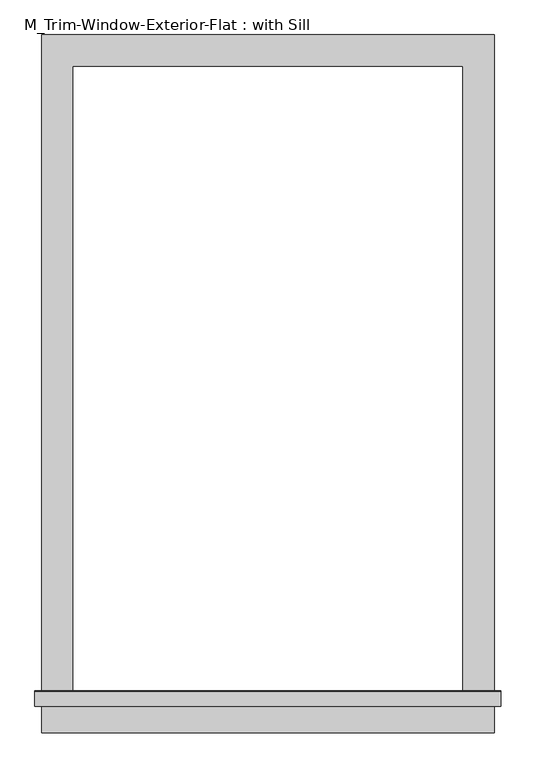
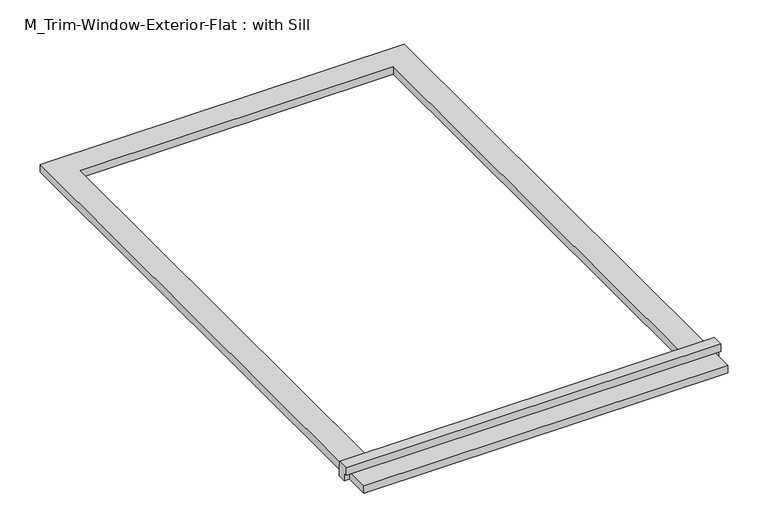
"""IFC4 building model written with IfcOpenShell, lengths in millimetres: proxy geometry, M_Trim-Window-Exterior-Flat : with Sill."""

from ifc_helpers import new_model, si_unit, frame, origin, origin_with_axes, place, context, project, spatial, polyline, outline, extrude, source, transform, mapped, element, save


def m_trim_window_exterior_flat_with_sill_e7ff6350(model_context):
    return source(origin(), model_context, "Body", "SweptSolid", [
        extrude(outline(polyline([(435.0, -1220.4323709), (435.0, -1280.4323709), (-435.0, -1280.4323709), (-435.0, -1220.4323709), (435.0, -1220.4323709)])), origin_with_axes(), (0.0, 0.0, 1.0), 19.05),
        extrude(outline(polyline([(-1230.0, 38.1), (-1202.4580645, 38.1), (-1200.0, 19.05), (-1200.0, 0.0), (-1220.4323709, 0.0), (-1220.4323709, 19.05), (-1230.0, 19.05), (-1230.0, 38.1)])), frame((-447.7, 0.0, 0.0), z_axis=(1.0, 0.0, 0.0), x_axis=(0.0, 1.0, 0.0)), (0.0, 0.0, 1.0), 895.4),
        extrude(outline(polyline([(-435.0, 60.0), (435.0, 60.0), (435.0, -1200.0), (375.0, -1200.0), (375.0, 0.0), (-375.0, 0.0), (-375.0, -1200.0), (-435.0, -1200.0), (-435.0, 60.0)])), origin_with_axes(), (0.0, 0.0, 1.0), 19.05),
    ])


if __name__ == "__main__":
    model = new_model("IFC4")
    model_context = context("Model", 3, world=origin())
    ifc_project = project(units=[si_unit("LENGTHUNIT", "METRE", prefix="MILLI")], contexts=[model_context])
    site = spatial("IfcSite", under=ifc_project)
    building = spatial("IfcBuilding", under=site)
    placement = place(None, origin())
    m_trim_window_exterior_flat_with_sill_shape = m_trim_window_exterior_flat_with_sill_e7ff6350(model_context)
    element("IfcBuildingElementProxy", 1, Name="M_Trim-Window-Exterior-Flat : with Sill", ObjectType="M_Trim-Window-Exterior-Flat : with Sill", at=placement, inside=building, context=model_context, shape_type="MappedRepresentation", body=[
        mapped(m_trim_window_exterior_flat_with_sill_shape, transform((0.0, 0.0, 0.0), x_axis=(1.0, 0.0, 0.0), y_axis=(0.0, 1.0, 0.0), z_axis=(0.0, 0.0, 1.0))),
    ])
    save(model, "model.ifc")

# Revit data of these elements
# Type "M_Trim-Window-Exterior-Flat : with Sill"
#   Trim Width = 0.06 m
#   Trim Thickness_Picture Frame = 0.03 m
#   Trim Thickness_with Sill = 0.01905 m
#   Sill Thickness = 0.03 m
#   Opening Width [instance default] = 0.6 m
#   Opening Height [instance default] = 0.9 m
#   Default Elevation = 1.2 m
#   Sill = yes
#   Picture Frame = no
#   Trim Material [instance default] = none
# Element 1 (IfcBuildingElementProxy, "M_Trim-Window-Exterior-Flat : with Sill")
#   Opening Width = 0.75 m
#   Opening Height = 1.2 m
#   Trim Material = Clad - White
#   Materials on its faces: "Clad - White"
# Materials
#   "Clad - White": class "Wood", colour RGB 242 242 238, transparency 0, Cost = 0
